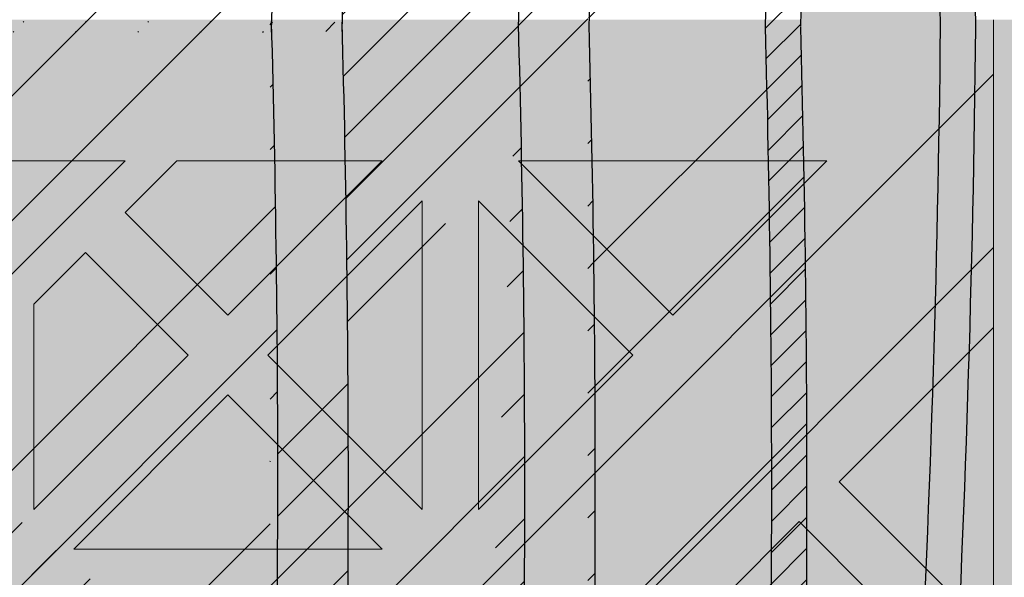
# Model space of a CAD drawing. Units: inches. Extents: x 844 to 2234, y 346 to 1084.
# Tile 54 of 93: x 1869.404 to 1873.853, y 698.846 to 701.365. Entities that reach past the tile are written whole.
import ezdxf

# ---------------------------------------------------------------- set-up
doc = ezdxf.new("R2010")
doc.units = ezdxf.units.IN
doc.header["$MEASUREMENT"] = 0
doc.layers.add('furniture', color=8, linetype='Continuous', lineweight=18)
doc.layers.add('RA-AP-01$0$INT', color=35, linetype='Continuous', lineweight=5)
doc.layers.add('RA-AP-01$0$FURN', color=3, linetype='Continuous')
doc.layers.add('RA-AP-01$0$WOOD', color=64, linetype='Continuous')

# ---------------------------------------------------------------- blocks, each defined once
blk = doc.blocks.new('A$C18D01794')
at = {"layer": 'RA-AP-01$0$INT'}
blk.add_hatch(color=256, dxfattribs=at).paths.add_polyline_path([(4.505206456958071, -6.306712009588038), (5.305206456958072, -6.306712009588038), (5.305206456958072, -7.106712009588038), (5.255206456951893, -7.10671200958804), (5.25520645694868, -6.356712009605972), (4.555206456959269, -6.356712009587461), (4.555206456956052, -7.106712009588038), (4.505206456958073, -7.106712009588038)])
h = blk.add_hatch(color=256, dxfattribs=at)
h.paths.add_polyline_path([(4.585917135068449, -6.356712009588271), (4.555206456959269, -6.35671200958746), (4.555206456959137, -6.387422687716308), (4.874495778835233, -6.706712009592356), (4.90520645695423, -6.676001331474049)])
h.paths.add_polyline_path([(5.255206456948813, -6.387422687716306), (5.255206456948682, -6.356712009605972), (5.224495778822613, -6.356712009605161), (4.905206456953498, -6.676001331474273), (4.935917135072151, -6.706712009592924)])
h.paths.add_polyline_path([(4.935917135072559, -6.706712009592068), (4.905206456953564, -6.737422687710376), (5.255206456951813, -7.087422687708613), (5.255206456951549, -7.026001331471008)])
h.paths.add_polyline_path([(4.555206456956399, -7.026001331471013), (4.555206456956134, -7.087422687708616), (4.905206456953821, -6.737422687710943), (4.874495778835166, -6.70671200959229)])
h = blk.add_hatch(color=256, dxfattribs=at)
h.paths.add_polyline_path([(4.585917135068448, -6.356712009588273), (4.614201406330596, -6.356712009589021), (4.668846067270487, -6.411356670531338), (4.723490728212344, -6.356712009591912), (4.771774999457151, -6.35671200959319), (4.826419660396886, -6.411356670535356), (4.862780050090322, -6.374996280843536), (4.844495778842715, -6.356712009595112), (4.862780050090411, -6.356712009595595), (4.905206456960182, -6.399138416468211), (4.947632863832445, -6.356712009597838), (4.965917135079675, -6.356712009598322), (4.947632863831759, -6.374996280845421), (4.983993253523576, -6.411356670538857), (5.038637914464627, -6.356712009600247), (5.08692218571208, -6.356712009601523), (5.141566846649976, -6.411356670541852), (5.196211507589851, -6.356712009604411), (5.224495778822615, -6.356712009605161), (4.905206456953975, -6.676001331473793)])
h.paths.add_polyline_path([(4.895206456956031, -6.637717060225675), (4.895206456958921, -6.528427738347902), (4.840561796018589, -6.583072399285802)], flags=16)
h.paths.add_polyline_path([(4.915206456955638, -6.637717060226121), (4.969851117895509, -6.583072399288678), (4.915206456957609, -6.528427738348344)], flags=16)
h.paths.add_polyline_path([(4.826419660395175, -6.568930263661755), (4.881064321335613, -6.514285602723745), (4.771774999456703, -6.514285602720857)], flags=16)
h.paths.add_polyline_path([(4.983993253519558, -6.568930263665262), (5.038637914460456, -6.514285602726792), (4.929348592581548, -6.514285602724816)], flags=16)
h.paths.add_polyline_path([(4.881064321336025, -6.494285602723742), (4.826419660397532, -6.439640941782821), (4.771774999457062, -6.494285602720859)], flags=16)
h.paths.add_polyline_path([(4.929348592582019, -6.494285602724817), (5.038637914460982, -6.494285602726792), (4.983993253522945, -6.439640941786327)], flags=16)
h.paths.add_polyline_path([(4.895206456960191, -6.480143467100443), (4.895206456962115, -6.407422687715913), (4.876922185715016, -6.389138416467584), (4.840561796021581, -6.425498806159401)], flags=16)
h.paths.add_polyline_path([(4.915206456958487, -6.480143467100889), (4.969851117899527, -6.425498806162279), (4.933490728206909, -6.389138416468043), (4.9152064569598, -6.40742268771434)], flags=16)
h.paths.add_polyline_path([(4.757632863832376, -6.480143467096812), (4.812277524772842, -6.425498806158772), (4.757632863834348, -6.370854145217844)], flags=16)
h.paths.add_polyline_path([(4.737632863832376, -6.480143467096286), (4.737632863834348, -6.370854145217375), (4.682988202893906, -6.425498806155385)], flags=16)
h.paths.add_polyline_path([(5.05278005008503, -6.480143467103376), (5.052780050087917, -6.370854145224413), (4.998135389146995, -6.425498806162908)], flags=16)
h.paths.add_polyline_path([(5.072780050085024, -6.480143467103744), (5.127424711025931, -6.42549880616527), (5.072780050087916, -6.370854145224832)], flags=16)
h.paths.add_polyline_path([(4.935917135072783, -6.706712009592292), (5.255206456948811, -6.387422687716309), (5.255206456948932, -6.415706958964177), (5.200561796010279, -6.470351619902839), (5.255206456949403, -6.524996280841948), (5.25520645694961, -6.5732805520894), (5.200561796009787, -6.627925213029239), (5.236922185702417, -6.664285602721864), (5.255206456949919, -6.646001331474357), (5.255206456949998, -6.664285602721898), (5.212780050078687, -6.706712009592262), (5.25520645695036, -6.749138416463932), (5.255206456950438, -6.767422687711313), (5.236922185702424, -6.749138416463297), (5.200561796009796, -6.785498806155928), (5.255206456950753, -6.840143467096874), (5.25520645695096, -6.888427738341682), (5.200561796010322, -6.943072399282328), (5.255206456951428, -6.997717060223427), (5.255206456951547, -7.026001331471006)])
h.paths.add_polyline_path([(5.042988202883395, -6.785498806155427), (5.097632863823085, -6.840143467095101), (5.097632863822622, -6.730854145216193)], flags=16)
h.paths.add_polyline_path([(5.028846067259663, -6.771356670531693), (5.083490728198774, -6.716712009592573), (4.974201406321001, -6.716712009593042)], flags=16)
h.paths.add_polyline_path([(5.117632863823087, -6.840143467095186), (5.172277524762331, -6.785498806155926), (5.11763286382262, -6.730854145216225)], flags=16)
h.paths.add_polyline_path([(5.08349072819877, -6.696712009593886), (5.028846067259652, -6.642067348654775), (4.974201406320998, -6.696712009593438)], flags=16)
h.paths.add_polyline_path([(5.131774999446817, -6.854285602718917), (5.186419660386065, -6.799640941779662), (5.241064321325782, -6.854285602719365)], flags=17)
h.paths.add_polyline_path([(5.131774999446228, -6.716712009592374), (5.186419660386065, -6.771356670532194), (5.222780050079488, -6.734996280838764), (5.204495778832781, -6.716712009592063)], flags=16)
h.paths.add_polyline_path([(5.097632863822613, -6.682569873970264), (5.097632863823061, -6.573280552091354), (5.042988202883383, -6.627925213031044)], flags=16)
h.paths.add_polyline_path([(5.131774999446899, -6.874285602718915), (5.241064321325809, -6.874285602719364), (5.186419660386591, -6.928930263658598)], flags=17)
h.paths.add_polyline_path([(5.131774999446226, -6.696712009594078), (5.204495778830767, -6.696712009594374), (5.22278005007868, -6.67842773834687), (5.186419660386049, -6.642067348654249)], flags=16)
h.paths.add_polyline_path([(5.11763286382262, -6.682569873970225), (5.17227752476232, -6.627925213030515), (5.117632863823064, -6.573280552091267)], flags=16)
h.paths.add_polyline_path([(5.186419660386069, -6.613783077405491), (5.241064321325754, -6.559138416465795), (5.131774999446791, -6.559138416466263)], flags=16)
h.paths.add_polyline_path([(5.131774999446872, -6.539138416466263), (5.24106432132578, -6.539138416465794), (5.186419660386554, -6.484493755526573)], flags=16)
h.paths.add_polyline_path([(5.255206456951811, -7.08742268770861), (5.255206456951895, -7.106712009588038), (4.555206456956052, -7.106712009588038), (4.555206456956136, -7.087422687708617), (4.905206456953973, -6.737422687710788)])
h.paths.add_polyline_path([(4.983993253513404, -6.8444937555241), (4.92934859257295, -6.899138416462108), (5.03863791445186, -6.899138416465014)], flags=16)
h.paths.add_polyline_path([(4.969851117889988, -6.83035161990006), (4.915206456952556, -6.775706958960171), (4.915206456949648, -6.884996280837944)], flags=16)
h.paths.add_polyline_path([(4.929348592572535, -6.919138416462105), (4.983993253511019, -6.973783077403037), (5.038637914451496, -6.919138416465012)], flags=16)
h.paths.add_polyline_path([(5.052780050074912, -6.93328055208906), (4.998135389134438, -6.987925213027088), (5.052780050072919, -7.042569873968025)], flags=16)
h.paths.add_polyline_path([(5.07278005007491, -6.933280552089588), (5.072780050072918, -7.042569873968497), (5.127424711013374, -6.987925213030498)], flags=16)
h.paths.add_polyline_path([(4.89520645695295, -6.775706958959721), (4.840561796013067, -6.830351619897157), (4.895206456950961, -6.884996280837494)], flags=16)
h.paths.add_polyline_path([(4.915206456948365, -6.933280552085403), (4.915206456946434, -7.006001331471951), (4.933490728192729, -7.024285602719066), (4.969851117886972, -6.987925213026453)], flags=16)
h.paths.add_polyline_path([(4.881064321327021, -6.899138416461022), (4.82641966038902, -6.84449375552057), (4.771774999448108, -6.899138416459029)], flags=16)
h.paths.add_polyline_path([(4.895206456950073, -6.933280552084951), (4.840561796009022, -6.987925213023558), (4.876922185700835, -7.024285602716997), (4.895206456948749, -7.006001331469487)], flags=16)
h.paths.add_polyline_path([(4.983993253510392, -7.0020673486505), (4.947632863816944, -7.038427738342319), (4.965917135064043, -7.05671200959023), (5.038637914448995, -7.056712009591555)], flags=16)
h.paths.add_polyline_path([(4.881064321326543, -6.91913841646102), (4.771774999447578, -6.919138416459031), (4.826419660385607, -6.973783077399508)], flags=16)
h.paths.add_polyline_path([(4.905206456946447, -7.014285602717636), (4.862780050074785, -7.056712009588352), (4.947632863816685, -7.056712009589775)], flags=16)
h.paths.add_polyline_path([(5.14156684663679, -7.002067348654549), (5.086922185696452, -7.056712009592438), (5.196211507574223, -7.056712009594425)], flags=16)
h.paths.add_polyline_path([(4.8264196603837, -7.002067348646972), (4.771774999442643, -7.056712009585575), (4.8444957788276, -7.056712009587508), (4.862780050075511, -7.038427738340416)], flags=16)
h.paths.add_polyline_path([(4.812277524760289, -6.98792521302292), (4.757632863822258, -6.933280552082447), (4.757632863819352, -7.042569873961408)], flags=16)
h.paths.add_polyline_path([(4.73763286382226, -6.933280552082079), (4.682988202881349, -6.987925213020536), (4.737632863819352, -7.04256987396099)], flags=16)
h.paths.add_polyline_path([(4.723490728195188, -7.056712009584289), (4.668846067257299, -7.002067348643949), (4.614201406317417, -7.056712009581383)], flags=16)
h.paths.add_polyline_path([(4.597632863829262, -6.706712009592262), (4.555206456957951, -6.664285602721896), (4.555206456958029, -6.646001331474357), (4.573490728205535, -6.664285602721864), (4.609851117898167, -6.627925213029238), (4.555206456958338, -6.573280552089402), (4.555206456958546, -6.524996280841952), (4.60985111789767, -6.470351619902839), (4.555206456959015, -6.415706958964177), (4.555206456959138, -6.387422687716309), (4.874495778835167, -6.70671200959229), (4.5552064569564, -7.026001331471015), (4.555206456956523, -6.997717060223433), (4.609851117897629, -6.94307239928233), (4.555206456956988, -6.888427738341681), (4.555206456957198, -6.840143467096881), (4.609851117898153, -6.78549880615593), (4.573490728205528, -6.749138416463297), (4.555206456957507, -6.76742268771132), (4.555206456957585, -6.749138416463933)])
h.paths.add_polyline_path([(4.712780050085332, -6.730854145216195), (4.712780050084863, -6.840143467095105), (4.767424711024555, -6.785498806155427)], flags=16)
h.paths.add_polyline_path([(4.726922185709173, -6.716712009592573), (4.781566846648288, -6.771356670531693), (4.836211507586949, -6.716712009593043)], flags=16)
h.paths.add_polyline_path([(4.692780050085327, -6.730854145216225), (4.638135389145619, -6.785498806155928), (4.692780050084865, -6.840143467095185)], flags=16)
h.paths.add_polyline_path([(4.726922185709182, -6.696712009593886), (4.836211507586949, -6.696712009593436), (4.7815668466483, -6.642067348654773)], flags=16)
h.paths.add_polyline_path([(4.678637914461726, -6.71671200959237), (4.605917135075169, -6.716712009592063), (4.587632863828464, -6.734996280838766), (4.623993253521887, -6.771356670532195)], flags=16)
h.paths.add_polyline_path([(4.712780050085336, -6.68256987397026), (4.767424711024568, -6.627925213031042), (4.71278005008489, -6.573280552091352)], flags=16)
h.paths.add_polyline_path([(4.678637914461726, -6.696712009594076), (4.623993253521899, -6.642067348654247), (4.587632863829271, -6.67842773834687), (4.605917135077185, -6.696712009594376)], flags=16)
h.paths.add_polyline_path([(4.692780050085336, -6.682569873970228), (4.692780050084889, -6.573280552091267), (4.638135389145632, -6.627925213030515)], flags=16)
h.paths.add_polyline_path([(4.623993253521885, -6.799640941779662), (4.678637914461131, -6.854285602718915), (4.56934859258217, -6.854285602719365)], flags=17)
h.paths.add_polyline_path([(4.623993253521901, -6.613783077405509), (4.678637914461158, -6.559138416466263), (4.569348592582195, -6.559138416465795)], flags=16)
h.paths.add_polyline_path([(4.678637914461051, -6.874285602718915), (4.623993253521361, -6.928930263658598), (4.569348592582143, -6.874285602719364)], flags=17)
h.paths.add_polyline_path([(4.678637914461076, -6.539138416466263), (4.623993253521399, -6.484493755526573), (4.569348592582167, -6.539138416465796)], flags=16)
h = blk.add_hatch(color=256, dxfattribs=at)
h.paths.add_polyline_path([(5.028846067259997, -6.642067348655121), (4.974201406321342, -6.696712009593783), (5.083490728199115, -6.69671200959423)])
h.paths.add_polyline_path([(4.974201406321344, -6.716712009593388), (5.028846067260004, -6.771356670532039), (5.083490728199117, -6.716712009592919)])
h.paths.add_polyline_path([(5.042988202883738, -6.785498806155768), (5.097632863823428, -6.840143467095449), (5.097632863822963, -6.73085414521654)])
h.paths.add_polyline_path([(5.117632863822961, -6.730854145216568), (5.117632863823428, -6.840143467095531), (5.172277524762674, -6.785498806156272)])
h.paths.add_polyline_path([(5.131774999446572, -6.716712009592718), (5.186419660386406, -6.77135667053254), (5.222780050079831, -6.734996280839116), (5.204495778833122, -6.716712009592409)])
h.paths.add_polyline_path([(5.236922185702764, -6.749138416463644), (5.200561796010139, -6.785498806156274), (5.255206456949971, -6.840143467096101), (5.255206456950271, -6.76742268771115)])
h.paths.add_polyline_path([(5.186419660386412, -6.799640941780006), (5.131774999447164, -6.854285602719262), (5.241064321326123, -6.854285602719711)])
h.paths.add_polyline_path([(5.131774999447238, -6.874285602719261), (5.186419660386934, -6.928930263658944), (5.241064321326153, -6.874285602719709)])
h.paths.add_polyline_path([(5.200561796010663, -6.943072399282675), (5.255206456949324, -6.997717060221329), (5.255206456949777, -6.888427738343558)])
h.paths.add_polyline_path([(5.21278005007903, -6.706712009592607), (5.255206456950223, -6.749138416463798), (5.255206456950696, -6.664285602721891)])
h.paths.add_polyline_path([(5.13177499944657, -6.696712009594424), (5.204495778831106, -6.696712009594723), (5.222780050079024, -6.678427738347219), (5.186419660386397, -6.642067348654592)])
h.paths.add_polyline_path([(5.117632863823405, -6.573280552091611), (5.117632863822955, -6.682569873970578), (5.172277524762665, -6.627925213030859)])
h.paths.add_polyline_path([(5.042988202883727, -6.627925213031387), (5.097632863822957, -6.682569873970603), (5.097632863823407, -6.573280552091697)])
h.paths.add_polyline_path([(5.131774999447135, -6.559138416466609), (5.186419660386394, -6.613783077405857), (5.241064321326097, -6.559138416466144)])
h.paths.add_polyline_path([(5.200561796010128, -6.627925213029584), (5.236922185702758, -6.664285602722211), (5.255206456950264, -6.646001331474705), (5.255206456949948, -6.573280552089752)])
h.paths.add_polyline_path([(5.186419660386895, -6.484493755526919), (5.131774999447213, -6.539138416466609), (5.241064321326127, -6.539138416466142)])
h.paths.add_polyline_path([(5.200561796010624, -6.470351619903183), (5.255206456949745, -6.524996280842298), (5.255206456949276, -6.415706958964523)])
h = blk.add_hatch(color=256, dxfattribs=at)
h.paths.add_polyline_path([(4.895206456952951, -6.77570695895972), (4.840561796013068, -6.830351619897156), (4.895206456950958, -6.884996280837495)])
h.paths.add_polyline_path([(4.915206456949649, -6.884996280837942), (4.969851117889987, -6.830351619900054), (4.915206456952556, -6.775706958960171)])
h.paths.add_polyline_path([(5.038637914451862, -6.899138416465013), (4.983993253513403, -6.8444937555241), (4.929348592572953, -6.899138416462106)])
h.paths.add_polyline_path([(4.929348592572535, -6.919138416462105), (4.983993253511018, -6.973783077403037), (5.038637914451497, -6.919138416465012)])
h.paths.add_polyline_path([(4.915206456948366, -6.933280552085397), (4.915206456946433, -7.006001331471951), (4.93349072819273, -7.024285602719068), (4.969851117886972, -6.987925213026454)])
h.paths.add_polyline_path([(5.038637914448995, -7.056712009591553), (4.983993253510389, -7.002067348650502), (4.947632863816946, -7.038427738342318), (4.965917135064043, -7.05671200959023)])
h.paths.add_polyline_path([(5.05278005007292, -7.042569873968023), (5.05278005007491, -6.933280552089059), (4.998135389134438, -6.987925213027088)])
h.paths.add_polyline_path([(5.07278005007292, -7.042569873968496), (5.127424711013374, -6.987925213030498), (5.072780050074909, -6.933280552089588)])
h.paths.add_polyline_path([(5.141566846636789, -7.002067348654547), (5.086922185696449, -7.056712009592438), (5.196211507574223, -7.056712009594425)])
h.paths.add_polyline_path([(4.947632863816688, -7.056712009589774), (4.905206456946449, -7.014285602717634), (4.862780050074784, -7.056712009588353)])
h.paths.add_polyline_path([(4.840561796009025, -6.987925213023556), (4.876922185700834, -7.024285602716997), (4.895206456948747, -7.006001331469488), (4.895206456950075, -6.933280552084953)])
h.paths.add_polyline_path([(4.88106432132654, -6.919138416461021), (4.771774999447577, -6.919138416459031), (4.826419660385606, -6.973783077399508)])
h.paths.add_polyline_path([(4.881064321327019, -6.899138416461022), (4.826419660389019, -6.844493755520571), (4.771774999448108, -6.89913841645903)])
h.paths.add_polyline_path([(4.757632863819352, -7.042569873961409), (4.812277524760284, -6.987925213022922), (4.757632863822259, -6.933280552082447)])
h.paths.add_polyline_path([(4.8264196603837, -7.002067348646974), (4.771774999442646, -7.056712009585575), (4.844495778827599, -7.05671200958751), (4.862780050075512, -7.038427738340417)])
h.paths.add_polyline_path([(4.737632863819352, -7.042569873960988), (4.737632863822258, -6.933280552082078), (4.682988202881349, -6.987925213020538)])
h.paths.add_polyline_path([(4.668846067257299, -7.002067348643952), (4.61420140631742, -7.056712009581384), (4.723490728195189, -7.056712009584292)])
for p, q in [((5.255206456951895, -7.106712009588038), (5.255206456948681, -6.356712009605972)), ((4.935917135072783, -6.706712009592292), (5.255206456951548, -7.026001331471007)), ((4.905206456953975, -6.737422687710788), (5.255206456951811, -7.087422687708611)), ((5.186419660386587, -6.928930263658596), (5.131774999446899, -6.874285602718915)), ((5.241064321325809, -6.874285602719364), (5.186419660386589, -6.928930263658598)), ((5.255206456949429, -6.888427738343214), (5.200561796010322, -6.943072399282328)), ((5.255206456949433, -6.888427738343212), (5.255206456948982, -6.997717060220983)), ((5.038637914451498, -6.919138416465012), (4.929348592572535, -6.919138416462105)), ((4.929348592572535, -6.919138416462105), (4.983993253511019, -6.973783077403037)), ((5.038637914451498, -6.919138416465012), (4.983993253511019, -6.973783077403037)), ((4.915206456946434, -7.006001331470351), (4.915206456948367, -6.933280552085399)), ((4.915206456948367, -6.933280552085399), (4.969851117886972, -6.987925213026453)), ((5.05278005007491, -6.93328055208906), (4.998135389134438, -6.987925213027088)), ((5.05278005007491, -6.93328055208906), (5.052780050072921, -7.042569873968023)), ((5.127424711013373, -6.987925213030496), (5.07278005007491, -6.933280552089588)), ((5.07278005007491, -6.933280552089588), (5.07278005007292, -7.042569873968497)), ((5.255206456948982, -6.997717060220983), (5.200561796010322, -6.943072399282328)), ((4.969851117886972, -6.987925213026452), (4.93349072819353, -7.024285602718265)), ((5.052780050072921, -7.042569873968023), (4.998135389134438, -6.987925213027088)), ((5.07278005007292, -7.042569873968497), (5.127424711013374, -6.987925213030498)), ((4.98399325351039, -7.002067348650502), (4.947632863816946, -7.038427738342317)), ((5.038637914448995, -7.056712009591555), (4.983993253510388, -7.002067348650502)), ((5.086922185696454, -7.056712009592434), (5.141566846636789, -7.002067348654547)), ((5.196211507574223, -7.056712009594425), (5.141566846636789, -7.002067348654547)), ((4.915206456946427, -7.006001331471944), (4.933490728193524, -7.02428560271986)), ((4.905206456946449, -7.014285602717635), (4.94763286381669, -7.056712009589775)), ((4.947632863816946, -7.038427738342317), (4.965917135063997, -7.056712009590183)), ((4.965917135064043, -7.056712009590231), (4.947632863816944, -7.038427738342317)), ((4.94763286381669, -7.056712009589775), (4.862780050074783, -7.056712009588354)), ((4.965917135064043, -7.05671200959023), (5.038637914448995, -7.056712009591555)), ((5.086922185696452, -7.056712009592438), (5.196211507574223, -7.056712009594425))]:
    blk.add_line(p, q, dxfattribs=at)
blk = doc.blocks.new('A$C32926AE1')
at = {"layer": 'RA-AP-01$0$FURN'}
h = blk.add_hatch(dxfattribs=at)
h.set_pattern_fill('ANSI31', color=256, scale=0.1, style=0)
h.set_pattern_definition([(45, (0, 0), (-0.0088388347648318, 0.0088388347648318), [])])
edge = h.paths.add_edge_path(flags=16)
edge.add_arc((4.904771284329206, 4.246793130718756), 0.2603971832811541, 75.22398030683196, 104.7760196931204)
edge.add_arc((4.904771284329206, 4.246793130718756), 0.2603971832811541, 75.223980306832, 104.77601969312039, ccw=False)
edge = h.paths.add_edge_path(flags=16)
edge.add_arc((4.904771284329206, 4.067062675376612), 0.2603971832811541, 255.2239803068796, 284.776019693168)
edge.add_arc((4.904771284329206, 4.067062675376612), 0.2603971832811541, 255.22398030687958, 284.77601969316805, ccw=False)
edge = h.paths.add_edge_path(flags=0)
edge.add_arc((4.904771284329206, 4.067062675376612), 0.2603971832811541, 255.2239803068796, 284.776019693168)
edge.add_arc((4.904771284329206, 4.067062675376612), 0.2603971832811541, 255.22398030687958, 284.77601969316805, ccw=False)
edge = h.paths.add_edge_path(flags=0)
edge.add_arc((4.904771284329206, 4.067062675376612), 0.2603971832811541, 255.2239803068796, 284.776019693168)
edge.add_arc((4.904771284329206, 4.067062675376612), 0.2603971832811541, 255.22398030687958, 284.77601969316805, ccw=False)
edge = h.paths.add_edge_path()
edge.add_arc((4.604388392048174, 4.588829985554312), 0.1599999999999918, 342.3781640246255, 354.4317409793762)
edge.add_arc((5.090145208887507, 4.43216705527679), 0.3503971832811637, 162.0091218307731, 180.3186872093483)
edge.add_arc((5.205154176610243, 4.588829985554953), 0.1599999999999917, 185.5682590208461, 197.6218359767349)
edge.add_arc((4.904771284329229, 4.246793130718735), 0.3503971832811761, 72.00912183053516, 107.9908781690354)
edge.add_arc((9.535952835716557, 4.28682295566602), 4.798342501046485, 178.2875002453811, 181.5576802719453)
edge.add_arc((4.719397359771122, 4.43216705527679), 0.3503971832811637, 359.6813127906516, 377.9908781692269)
edge.add_arc((9.535967292294904, 4.286822350292874), 4.778371420254705, 178.2965938931842, 181.5667745797229)
edge.add_arc((4.719397359771122, 4.43216705527679), 0.3303971832811637, 359.6813127906516, 377.9908781692269)
edge.add_arc((0.2735752763637294, 4.286822350292874), 4.7783714202547, 358.4332254202771, 361.7034061068158)
edge.add_arc((5.061434214606998, 4.732549947558029), 0.1600000000000254, 252.3781640250584, 264.4317409792362)
edge.add_arc((4.748108354051257, 4.732549947558012), 0.1600000000000541, 275.5682590208426, 287.6218359759532)
edge.add_arc((4.604388392048115, 4.588829985554317), 0.1800000000000505, 342.3567572500182, 349.3735009646207)
edge.add_arc((5.205154176610254, 4.588829985554976), 0.1800000000000069, 190.6264990356027, 197.6432427513933)
edge.add_arc((5.061434214607106, 4.732549947558013), 0.1800000000000424, 252.3567572496606, 259.3735009644582)
edge.add_arc((4.904771284329208, 4.246793130718737), 0.3303971832811676, 71.99844483668534, 108.0015551637021)
edge.add_arc((4.748108354051414, 4.732549947558045), 0.1800000000000547, 280.6264990355479, 287.6432427495938)
edge.add_arc((5.090145208887514, 4.432167055276789), 0.2803971832811691, 162.8706300666893, 180.816523289902)
edge.add_arc((4.719397359771136, 4.432167055276689), 0.2803971832811534, 359.183476710103, 377.1293699333214)
edge.add_arc((4.904771284329222, 4.246793130718737), 0.2803971832811769, 72.87063006672916, 107.1293699332334)
edge.add_arc((5.090145208887522, 4.432167055276788), 0.2603971832811776, 165.2239803068007, 180.9953123810312)
edge.add_arc((4.719397359771141, 4.432167055276699), 0.2603971832811458, 359.0046876189768, 374.7760196932087)
edge.add_arc((5.090145208887507, 4.43216705527679), 0.3303971832811637, 162.0091218307731, 180.3186872093483)
edge.add_arc((9.53595427642584, 4.285015535491528), 4.728345371032053, 178.265043920078, 181.5679956281801)
edge.add_arc((0.2735882922327999, 4.285015535491582), 4.728345371032045, 358.4320043718193, 361.7349560799204)
edge.add_arc((9.535953591267507, 4.284458026472751), 4.708343996644348, 178.2573054306777, 181.5704995759608)
edge.add_arc((0.273588977391114, 4.284458026472785), 4.708343996644358, 358.4295004240388, 361.7426945693213)
edge.add_arc((0.2735889773911131, 4.029397779622582), 4.708343996644359, 358.2573054306787, 361.5704995759613)
edge.add_arc((9.535953591267518, 4.029397779622618), 4.708343996644359, 178.4295004240391, 181.7426945693223)
edge.add_arc((0.2735882922327901, 4.028840270603786), 4.728345371032054, 358.2650439200796, 361.5679956281808)
edge.add_arc((9.53595427642584, 4.028840270603841), 4.728345371032054, 178.4320043718199, 181.7349560799219)
edge.add_arc((0.2735752763637302, 4.027033455802493), 4.778371420254699, 358.2965938931842, 361.5667745797229)
edge.add_arc((4.719397359771122, 3.881688750818578), 0.3303971832811637, 342.0091218307731, 360.3186872093484)
edge.add_arc((5.090145208887507, 3.881688750818578), 0.3303971832811637, 179.6813127906516, 197.9908781692269)
edge.add_arc((9.535967292294904, 4.027033455802493), 4.778371420254705, 178.433225420277, 181.7034061068158)
edge.add_arc((4.719397359771122, 3.881688750818578), 0.3503971832811637, 342.0091218307731, 360.3186872093484)
edge.add_arc((9.53595283571655, 4.027032850429349), 4.79834250104648, 178.4423197280546, 181.7124997546188)
edge.add_arc((4.719397359771141, 3.881688750818669), 0.2603971832811458, 345.2239803067913, 360.9953123810232)
edge.add_arc((5.090145208887522, 3.88168875081858), 0.2603971832811776, 179.0046876189687, 194.7760196931993)
edge.add_arc((4.904771284329222, 4.067062675376631), 0.2803971832811769, 252.8706300667665, 287.1293699332708)
edge.add_arc((4.719397359771136, 3.881688750818678), 0.2803971832811534, 342.8706300666787, 360.8165232898969)
edge.add_arc((5.090145208887514, 3.881688750818579), 0.2803971832811691, 179.183476710098, 197.1293699333106)
edge.add_arc((4.748108354051414, 3.581305858537323), 0.1800000000000547, 72.3567572504062, 79.37350096445199)
edge.add_arc((4.904771284329208, 4.067062675376631), 0.3303971832811676, 251.9984448362979, 288.0015551633146)
edge.add_arc((5.061434214607106, 3.581305858537355), 0.1800000000000424, 100.6264990355418, 107.6432427503394)
edge.add_arc((5.205154176610254, 3.725025820540392), 0.1800000000000069, 162.3567572486066, 169.3735009643972)
edge.add_arc((4.604388392048115, 3.725025820541051), 0.1800000000000505, 10.62649903537925, 17.64324274998182)
edge.add_arc((4.748108354051257, 3.581305858537356), 0.1600000000000541, 72.37816402404681, 84.43174097915735)
edge.add_arc((4.904771284329229, 4.067062675376632), 0.3503971832811761, 252.0091218309645, 287.9908781694648)
edge.add_arc((5.061434214606998, 3.581305858537339), 0.1600000000000254, 95.56825902076373, 107.6218359749416)
edge.add_arc((5.205154176610243, 3.725025820540414), 0.1599999999999917, 162.3781640232651, 174.4317409791539)
edge.add_arc((5.090145208887507, 3.881688750818578), 0.3503971832811637, 179.6813127906516, 197.9908781692269)
edge.add_arc((4.604388392048174, 3.725025820541056), 0.1599999999999918, 5.568259020623824, 17.62183597537444)
edge.add_arc((0.2735897329420762, 4.28682295566602), 4.798342501046482, 358.4423197280547, 361.7124997546188)
edge.add_arc((0.2735897329420691, 4.027032850429348), 4.798342501046489, 358.2875002453812, 361.5576802719453)
at = {"layer": 'RA-AP-01$0$WOOD'}
h = blk.add_hatch(color=256, dxfattribs=at)
h.dxf.hatch_style = 1
h.paths.add_polyline_path([(5.157430609644524, 4.573483066760929, -0.1009492694046607), (5.155401577623758, 4.593365984175333, -0.1842662638101597), (5.172249623284174, 4.638795604568598, 0.2056608120311276), (5.179560981299304, 4.661316324430096, 0.3614336704623542), (5.134352340494423, 4.706524965234944, 0.2056608120311297), (5.111831620632933, 4.699213607219793, -0.1842662638101113), (5.066402000239693, 4.682365561559342, -0.1055311479399994), (5.045656153913092, 4.68467289944697, 0.1567636581983829), (4.763886414745334, 4.684672899446966, -0.1055311479399895), (4.743140568418733, 4.68236556155934, -0.1842662638100833), (4.6977109480255, 4.69921360721979, 0.2056608120302612), (4.675190228164109, 4.706524965234949, 0.3614336704708441), (4.629981587358889, 4.66131632442871, 0.2056608120245944), (4.637292945374126, 4.638795604567974, -0.1842662638101024), (4.654140991034615, 4.59336598417475, -0.1009492694055169), (4.652111959013835, 4.573483066760181, 0.021410119221476), (4.629748025606143, 4.156712009541676, 0.0214101192214795), (4.652111959013809, 3.739940952323101, -0.1009492694059586), (4.654140991034615, 3.720058034908448, -0.1842662638100975), (4.637292945374126, 3.674628414515226, 0.2056608120245705), (4.629981587358889, 3.652107694654492, 0.3614336704708879), (4.675190228164113, 3.606899053848249, 0.2056608120302384), (4.697710948025501, 3.614210411863408, -0.1842662638100995), (4.743140568418738, 3.63105845752386, -0.1055311479402541), (4.763886414745388, 3.628751119636215, 0.1567636581983776), (5.045656153913137, 3.628751119636244, -0.1055311479397538), (5.066402000239692, 3.631058457523857, -0.1842662638101067), (5.111831620632931, 3.614210411863407, 0.2056608120310924), (5.134352340494417, 3.606899053848256, 0.3614336704624001), (5.179560981299307, 3.652107694653103, 0.2056608120311314), (5.172249623284175, 3.6746284145146, -0.1842662638101402), (5.155401577623758, 3.72005803490786, -0.1009492694051366), (5.15743060964455, 3.739940952322354, 0.0214101192215073), (5.179794543052287, 4.156712009541468, 0.0214101192215252)])
h.paths.add_polyline_path([(4.639748609479751, 4.156712009541513, 0.0213537860821624), (4.661970494867118, 3.741887061152232, -0.094075836301374), (4.664143710413708, 3.7196126951003, -0.1824818158568985), (4.644813765429836, 3.668037719127816, 0.2056608120245319), (4.639939526753007, 3.653023905887301, 0.3614336704710246), (4.676106439397173, 3.616856993242342, 0.2056608120302234), (4.691120252638095, 3.621731231919122, -0.1824818158602558), (4.742695228611606, 3.641061176902986, -0.1029891339458722), (4.766991894714349, 3.638256818950944, 0.156709409989566), (5.042550673941472, 3.638256818950105, -0.102989133958497), (5.066847340047078, 3.641061176902949, -0.1824818158594995), (5.118422316020358, 3.621731231919103, 0.2056608120311416), (5.133436129261316, 3.616856993242346, 0.3614336704621468), (5.169603041905217, 3.653023905886178, 0.2056608120310986), (5.164728803228477, 3.668037719127177, -0.1824818158565612), (5.145398858244737, 3.719612695099578, -0.0940758363009313), (5.147572073791232, 3.741887061151398, 0.0213537860822023), (5.169793959178681, 4.156712009541451, 0.0213537860822226), (5.147572073791203, 4.571536957931898, -0.0940758363005034), (5.145398858244737, 4.59381132398362, -0.1824818158565587), (5.164728803228476, 4.645386299956021, 0.2056608120311045), (5.169603041905216, 4.66040011319702, 0.3614336704621845), (5.133436129261313, 4.696567025840856, 0.2056608120310773), (5.118422316020359, 4.691692787164098, -0.182481815859508), (5.066847340047078, 4.67236284218025, -0.1029891339584606), (5.04255067394148, 4.675167200133092, 0.156709409989566), (4.766991894714357, 4.675167200132257, -0.1029891339458842), (4.742695228611611, 4.672362842180213, -0.1824818158602725), (4.691120252638095, 4.691692787164077, 0.2056608120302152), (4.676106439397174, 4.696567025840858, 0.3614336704710363), (4.639939526753005, 4.660400113195899, 0.2056608120245495), (4.644813765429837, 4.645386299955384, -0.1824818158568934), (4.664143710413708, 4.593811323982902, -0.0940758363009187), (4.661970494867149, 4.571536957931074, 0.021353786082177)], flags=16)
h.paths.add_polyline_path([(5.129794543052235, 4.432167055276933, -0.0141661062790638), (5.130152669293814, 4.156927903047693, -0.0141661062790647), (5.129794543052234, 3.881688750818433, -0.0785247771143638), (5.10979738006795, 3.755143611847103, 0.0945969212073497), (5.105408519571111, 3.717898134952927, 0.1043170707844957), (5.116074640131521, 3.670385395016088, 0.1043170707864965), (5.068561900193738, 3.681051515576561, 0.09459692119553), (5.031316423304057, 3.676662655080835, -0.1580239521427272), (4.778226145355827, 3.676662655080367, 0.0945969211986668), (4.740980668464973, 3.681051515576592, 0.1043170707882822), (4.693467928526415, 3.670385395015844, 0.1043170707867916), (4.704134049087309, 3.717898134953662, 0.0945969211972894), (4.69974518859162, 3.755143611844042, -0.0785247771163196), (4.679748025606343, 3.881688750818406, -0.0141661062790663), (4.679389899364763, 4.156927903047693, -0.0141661062790672), (4.679748025606343, 4.432167055276998, -0.0785247771163064), (4.699745188591625, 4.55871219425134, 0.094596921197333), (4.704134049087308, 4.595957671141738, 0.1043170707867205), (4.693467928526416, 4.643470411079523, 0.1043170707882628), (4.740980668464965, 4.632804290518776, 0.0945969211988114), (4.778226145355874, 4.637193151015016, -0.158023952142669), (5.031316423304015, 4.637193151014546, 0.0945969211956361), (5.068561900193736, 4.632804290518806, 0.1043170707864979), (5.11607464013152, 4.643470411079278, 0.1043170707844617), (5.105408519571112, 4.595957671142455, 0.0945969212074597), (5.109797380067959, 4.558712194248236, -0.0785247771143467)], flags=0)
h.paths.add_polyline_path([(5.119794532311105, 4.432259799204851, -0.0142000800617244), (5.120156169157484, 4.156927903047701, -0.0142000800617277), (5.119794532311105, 3.881596006890482, -0.0784894509520253), (5.100273383573699, 3.758192358677797, 0.0940138827242913), (5.095413455884425, 3.717477693979438, 0.0606271852308753), (5.099615656341024, 3.686844378806616, 0.0606271852322524), (5.068982341167493, 3.691046579263239, 0.0940138827010453), (5.028267676478798, 3.686186651576848, -0.1580706864508061), (4.781274892180912, 3.686186651576435, 0.0940138827026903), (4.740560227491556, 3.691046579263279, 0.0606271852339895), (4.709926912317155, 3.686844378806508, 0.0606271852329405), (4.714129112773991, 3.717477693980356, 0.094013882701304), (4.709269185087677, 3.758192358669163, -0.0784894509577193), (4.689748036347473, 3.881596006890469, -0.014200080061729), (4.689386399501094, 4.156927903047709, -0.0142000800617217), (4.689748036347473, 4.432259799204808, -0.078489450957724), (4.709269185087651, 4.555663447426125, 0.0940138827014585), (4.714129112773992, 4.596378112114996, 0.0606271852329731), (4.709926912317154, 4.62701142728886, 0.0606271852340196), (4.74056022749157, 4.622809226832087, 0.0940138827024997), (4.781274892180847, 4.627669154518912, -0.1580706864508359), (5.028267676478777, 4.627669154518526, 0.0940138827010946), (5.068982341167492, 4.622809226832129, 0.060627185232254), (5.099615656341024, 4.627011427288751, 0.0606271852308727), (5.095413455884425, 4.59637811211593, 0.0940138827241088), (5.100273383573675, 4.555663447417647, -0.0784894509520978)], flags=0)
h.paths.add_polyline_path([(5.06978912287499, 4.430218106756144, -0.014241683694547), (5.070173729147532, 4.156927903047672, -0.0142416836945458), (5.06978912287499, 3.883637699339223, -0.0800609523125196), (5.052662118612511, 3.773463122773442, 0.0526421978001116), (5.04590916754064, 3.740550867606997, 0.0526421977992423), (5.012996912374707, 3.73379791653534, -0.1583028414718258), (4.796545656286308, 3.73379791653451, 0.0526421978034211), (4.763633401117837, 3.740550867607021, 0.0526421978018622), (4.756880450045755, 3.773463122774558, -0.0800609523117106), (4.739753445783639, 3.883637699339268, -0.0142416836945435), (4.739368839511098, 4.156927903047671, -0.0142416836945477), (4.739753445783639, 4.430218106756155, -0.0800609523116345), (4.75688045004574, 4.540392683320762, 0.052642197801941), (4.763633401117837, 4.573304938488346, 0.0526421978035071), (4.796545656286361, 4.580057889560873, -0.1583028414717561), (5.012996912374669, 4.580057889560039, 0.0526421977993048), (5.04590916754064, 4.57330493848837, 0.0526421978002057), (5.052662118612529, 4.540392683321868, -0.080060952312477)], flags=0)
h.paths.add_polyline_path([(5.049789715110557, 4.43038092723357, -0.0143097550741839), (5.05018085590259, 4.156927903047715, -0.0143097550741854), (5.049789715110558, 3.883474878861827, -0.0800685599149176), (5.03362098255317, 3.779581877367999, 0.0306258898956367), (5.028241146483733, 3.758218888663947, 0.0306258898977031), (5.006878157778253, 3.75283905259408, -0.1583983521624096), (4.802664410878162, 3.752839052594731, 0.0306258898946014), (4.781301422174808, 3.758218888663924, 0.0306258898967912), (4.775921586105202, 3.779581877368794, -0.080068559914251), (4.759752853548071, 3.883474878861786, -0.0143097550741854), (4.759361712756037, 4.156927903047671, -0.0143097550741854), (4.759752853548071, 4.430380927233557, -0.0800685599142479), (4.775921586105193, 4.534273928726546, 0.0306258898968306), (4.781301422174808, 4.555636917431444, 0.0306258898945754), (4.802664410878143, 4.561016753500631, -0.1583983521624168), (5.006878157778244, 4.561016753501291, 0.0306258898977177), (5.028241146483733, 4.555636917431421, 0.0306258898958182), (5.03362098255321, 4.534273928727244, -0.080068559914796)], flags=0)
h.paths.add_polyline_path([(4.999766070382627, 4.428171244713864, -0.0143443147609634), (5.000198441819402, 4.156927903047689, -0.0143443147609612), (4.999766070382627, 3.885684561381556, -0.0784641635803329), (4.987356730658798, 3.799103304488872, -0.1506053783831347), (4.822185837999821, 3.79910330448882, -0.0784641635803318), (4.809776498276007, 3.885684561381509, -0.014344314760963), (4.809344126839227, 4.156927903047677, -0.0143443147609645), (4.809776498276007, 4.428171244713873, -0.0784641635803192), (4.822185837999822, 4.514752501606549, -0.1506053783831338), (4.987356730658798, 4.514752501606494, -0.078464163580285)], flags=0)
h.paths.add_polyline_path([(4.979755254238824, 4.42764379880488, -0.0143772539198268), (4.980205517789977, 4.156927903047693, -0.0143772539198275), (4.979755254238824, 3.886212007290489, -0.0689242507424422), (4.971183264704897, 3.815276770442801, -0.1296645318904179), (4.838359303953726, 3.815276770442746, -0.0689242507424186), (4.829787314419809, 3.886212007290419, -0.0143772539198292), (4.829337050868653, 4.156927903047653, -0.0143772539198325), (4.829787314419809, 4.427643798804946, -0.0689242507424211), (4.838359303953725, 4.498579035652621, -0.1296645318904187), (4.971183264704897, 4.498579035652565, -0.0689242507424401)], flags=0)
h = blk.add_hatch(color=256, dxfattribs=at)
h.dxf.hatch_style = 1
h.paths.add_polyline_path([(5.145398858244737, 4.59381132398362, -0.1824818158565616), (5.164728803228476, 4.645386299956021, 0.2056608120311045), (5.169603041905216, 4.66040011319702, 0.3614336704621845), (5.133436129261313, 4.696567025840856, 0.2056608120310773), (5.118422316020359, 4.691692787164098, -0.182481815859508), (5.066847340047078, 4.67236284218025, -0.1029891339584606), (5.04255067394148, 4.675167200133092, 0.156709409989566), (4.766991894714357, 4.675167200132257, -0.1029891339458842), (4.742695228611611, 4.672362842180213, -0.1824818158602725), (4.691120252638095, 4.691692787164077, 0.2056608120302152), (4.676106439397174, 4.696567025840858, 0.3614336704710363), (4.639939526753005, 4.660400113195899, 0.2056608120245495), (4.644813765429837, 4.645386299955384, -0.1824818158568934), (4.664143710413708, 4.593811323982902, -0.0940758363009187), (4.661970494867149, 4.571536957931074, 0.0213537860821772), (4.639748609479751, 4.156712009541507, 0.0213537860821625), (4.661970494867119, 3.741887061152226, -0.0940758363013071), (4.664143710413708, 3.719612695100309, -0.1824818158569294), (4.644813765429836, 3.668037719127816, 0.2056608120245319), (4.639939526753007, 3.653023905887301, 0.3614336704710246), (4.676106439397173, 3.616856993242342, 0.2056608120302234), (4.691120252638095, 3.621731231919122, -0.1824818158602558), (4.742695228611606, 3.641061176902986, -0.1029891339458722), (4.766991894714349, 3.638256818950944, 0.156709409989566), (5.042550673941472, 3.638256818950105, -0.102989133958497), (5.066847340047078, 3.641061176902949, -0.1824818158594995), (5.118422316020358, 3.621731231919103, 0.2056608120311416), (5.133436129261316, 3.616856993242346, 0.3614336704621468), (5.169603041905217, 3.653023905886178, 0.2056608120310986), (5.164728803228477, 3.668037719127177, -0.1824818158565612), (5.145398858244737, 3.719612695099578, -0.0940758363009313), (5.147572073791232, 3.741887061151398, 0.0213537860822023), (5.169793959178681, 4.156712009541451, 0.0213537860822226), (5.147572073791203, 4.571536957931898, -0.0940758363004996)])
h.paths.add_polyline_path([(5.109797380067958, 4.55871219424824, -0.0785247771143472), (5.129794543052234, 4.432167055276936, -0.0141661062790644), (5.130152669293814, 4.156927903047685, -0.014166106279066), (5.129794543052234, 3.881688750818401, -0.0785247771143517), (5.109797380067946, 3.755143611847092, 0.0945969212073132), (5.105408519571111, 3.717898134952929, 0.1043170707844995), (5.116074640131521, 3.670385395016088, 0.1043170707864965), (5.068561900193738, 3.681051515576561, 0.09459692119553), (5.031316423304057, 3.676662655080835, -0.1580239521427272), (4.778226145355827, 3.676662655080367, 0.0945969211986668), (4.740980668464973, 3.681051515576592, 0.1043170707882822), (4.693467928526415, 3.670385395015844, 0.1043170707867916), (4.704134049087309, 3.717898134953662, 0.0945969211972894), (4.69974518859162, 3.755143611844042, -0.0785247771163196), (4.679748025606343, 3.881688750818406, -0.0141661062790663), (4.679389899364763, 4.156927903047693, -0.0141661062790672), (4.679748025606343, 4.432167055276998, -0.0785247771163064), (4.699745188591625, 4.55871219425134, 0.094596921197333), (4.704134049087308, 4.595957671141738, 0.1043170707867205), (4.693467928526416, 4.643470411079523, 0.1043170707882628), (4.740980668464965, 4.632804290518776, 0.0945969211988114), (4.778226145355874, 4.637193151015016, -0.158023952142669), (5.031316423304015, 4.637193151014546, 0.0945969211956361), (5.068561900193736, 4.632804290518806, 0.1043170707864979), (5.11607464013152, 4.643470411079278, 0.1043170707844617), (5.105408519571112, 4.595957671142455, 0.0945969212074504)], flags=16)
h.paths.add_polyline_path([(5.100273383573655, 4.55566344741771, -0.0784894509521388), (5.119794532311105, 4.432259799204852, -0.0142000800617252), (5.120156169157484, 4.156927903047686, -0.014200080061726), (5.119794532311105, 3.881596006890502, -0.0784894509520446), (5.100273383573696, 3.758192358677786, 0.0940138827242721), (5.095413455884425, 3.717477693979436, 0.0606271852308692), (5.099615656341024, 3.686844378806616, 0.0606271852322522), (5.068982341167493, 3.691046579263239, 0.0940138827010453), (5.028267676478798, 3.686186651576848, -0.1580706864508061), (4.781274892180912, 3.686186651576435, 0.0940138827026903), (4.740560227491556, 3.691046579263279, 0.0606271852339895), (4.709926912317155, 3.686844378806508, 0.0606271852329405), (4.714129112773991, 3.717477693980356, 0.094013882701304), (4.709269185087677, 3.758192358669163, -0.0784894509577193), (4.689748036347473, 3.881596006890469, -0.014200080061729), (4.689386399501094, 4.156927903047709, -0.0142000800617217), (4.689748036347473, 4.432259799204808, -0.078489450957724), (4.709269185087651, 4.555663447426125, 0.0940138827014585), (4.714129112773992, 4.596378112114996, 0.0606271852329731), (4.709926912317154, 4.62701142728886, 0.0606271852340196), (4.74056022749157, 4.622809226832087, 0.0940138827024997), (4.781274892180847, 4.627669154518912, -0.1580706864508359), (5.028267676478777, 4.627669154518526, 0.0940138827010946), (5.068982341167492, 4.622809226832129, 0.060627185232254), (5.099615656341024, 4.627011427288751, 0.0606271852308727), (5.095413455884425, 4.59637811211593, 0.094013882723957)], flags=0)
h.paths.add_polyline_path([(5.04590916754064, 4.57330493848837, 0.0526421978002057), (5.052662118612529, 4.540392683321868, -0.0800609523124783), (5.06978912287499, 4.430218106756142, -0.0142416836945469), (5.070173729147532, 4.156927903047672, -0.0142416836945458), (5.06978912287499, 3.883637699339223, -0.0800609523125196), (5.052662118612511, 3.773463122773442, 0.0526421978001116), (5.04590916754064, 3.740550867606997, 0.0526421977992423), (5.012996912374707, 3.73379791653534, -0.1583028414718258), (4.796545656286308, 3.73379791653451, 0.0526421978034211), (4.763633401117837, 3.740550867607021, 0.0526421978018622), (4.756880450045755, 3.773463122774558, -0.0800609523117106), (4.739753445783639, 3.883637699339268, -0.0142416836945435), (4.739368839511098, 4.156927903047671, -0.0142416836945477), (4.739753445783639, 4.430218106756155, -0.0800609523116345), (4.75688045004574, 4.540392683320762, 0.052642197801941), (4.763633401117837, 4.573304938488346, 0.0526421978035071), (4.796545656286361, 4.580057889560873, -0.1583028414717561), (5.012996912374669, 4.580057889560039, 0.0526421977993048)], flags=0)
h.paths.add_polyline_path([(5.028241146483733, 4.555636917431422, 0.0306258898956949), (5.033620982553182, 4.534273928727329, -0.0800685599148649), (5.049789715110557, 4.430380927233569, -0.0143097550741839), (5.05018085590259, 4.156927903047715, -0.0143097550741854), (5.049789715110558, 3.883474878861827, -0.0800685599149176), (5.03362098255317, 3.779581877367999, 0.0306258898956367), (5.028241146483733, 3.758218888663947, 0.0306258898977031), (5.006878157778253, 3.75283905259408, -0.1583983521624096), (4.802664410878162, 3.752839052594731, 0.0306258898946014), (4.781301422174808, 3.758218888663924, 0.0306258898967912), (4.775921586105202, 3.779581877368794, -0.080068559914251), (4.759752853548071, 3.883474878861786, -0.0143097550741854), (4.759361712756037, 4.156927903047671, -0.0143097550741854), (4.759752853548071, 4.430380927233557, -0.0800685599142479), (4.775921586105193, 4.534273928726546, 0.0306258898968306), (4.781301422174808, 4.555636917431444, 0.0306258898945754), (4.802664410878143, 4.561016753500631, -0.1583983521624168), (5.006878157778244, 4.561016753501291, 0.0306258898977174)], flags=0)
h.paths.add_polyline_path([(4.987356730658798, 4.514752501606494, -0.0784641635803018), (4.999766070382627, 4.428171244713845, -0.0143443147609637), (5.000198441819402, 4.156927903047665, -0.0143443147609622), (4.999766070382628, 3.885684561381514, -0.0784641635802952), (4.987356730658797, 3.799103304488872, -0.1506053783831338), (4.822185837999821, 3.799103304488819, -0.0784641635803342), (4.809776498276007, 3.885684561381512, -0.0143443147609628), (4.809344126839227, 4.156927903047676, -0.0143443147609646), (4.809776498276007, 4.428171244713873, -0.0784641635803192), (4.822185837999822, 4.514752501606549, -0.1506053783831338)], flags=0)
h.paths.add_polyline_path([(4.971183264704897, 4.498579035652566, -0.0689242507424384), (4.979755254238824, 4.427643798804883, -0.0143772539198276), (4.980205517789977, 4.15692790304768, -0.0143772539198258), (4.979755254238823, 3.88621200729051, -0.0689242507424628), (4.971183264704897, 3.815276770442801, -0.129664531890417), (4.838359303953726, 3.815276770442746, -0.0689242507424186), (4.829787314419809, 3.886212007290419, -0.0143772539198292), (4.829337050868653, 4.156927903047653, -0.0143772539198325), (4.829787314419809, 4.427643798804946, -0.0689242507424211), (4.838359303953725, 4.498579035652621, -0.1296645318904187)], flags=0)
h = blk.add_hatch(dxfattribs=at)
h.set_pattern_fill('ANSI31', color=256, scale=0.05, style=0)
h.set_pattern_definition([(45, (0, 0), (-0.0044194173824159, 0.0044194173824159), [])])
h.paths.add_polyline_path([(5.130152669293814, 4.156927903047704, 0.0141661062790657), (5.129794543052234, 4.432167055276982, 0.0777827904001433), (5.110168979996553, 4.557559993161921, -0.0976515123401879), (5.105408519571111, 4.595957671142454, -0.1043170707844687), (5.116074640131522, 4.64347041107928), (5.099615656341024, 4.627011427288751, 0.0606271852308727), (5.095413455884425, 4.59637811211593, 0.0940138827241088), (5.100273383573675, 4.555663447417647, -0.0784894509520972), (5.119794532311105, 4.432259799204852, -0.0142000800617252), (5.120156169157484, 4.156927903047686, -0.014200080061726), (5.119794532311105, 3.881596006890502, -0.0784894509520446), (5.100273383573696, 3.758192358677786, 0.0940138827242721), (5.095413455884425, 3.717477693979436, 0.0606271852308692), (5.099615656341024, 3.686844378806616), (5.116074640131519, 3.67038539501609, -0.1043170707844594), (5.105408519571112, 3.717898134952912, -0.0976515123401594), (5.11016897999655, 3.756295812933435, 0.0777827904001654), (5.129794543052234, 3.881688750818409, 0.0141661062790665)])
h.paths.add_polyline_path([(5.030164222210597, 3.676291055149937, -0.0976515123472002), (5.068561900193739, 3.681051515576561, -0.1043170707864927), (5.116074640131521, 3.670385395016088), (5.099615656341024, 3.686844378806616, 0.0606271852322522), (5.068982341167493, 3.691046579263239, 0.0940138827010453), (5.028267676478798, 3.686186651576848, -0.1580706864508061), (4.781274892180912, 3.686186651576435, 0.0940138827026903), (4.740560227491556, 3.691046579263279, 0.0606271852339913), (4.709926912317154, 3.686844378806508), (4.693467928526416, 3.670385395015845, -0.1043170707882796), (4.740980668464973, 3.681051515576592, -0.0976515123427246), (4.779378346446416, 3.676291055150394, 0.156512506893803)])
h.paths.add_polyline_path([(4.689748036347473, 3.881596006890472, -0.014200080061729), (4.689386399501094, 4.156927903047712, -0.0142000800617195), (4.689748036347473, 4.432259799204768, -0.078489450957742), (4.709269185087648, 4.555663447426114, 0.0940138827014821), (4.714129112773992, 4.596378112114995, 0.0606271852329748), (4.709926912317154, 4.62701142728886), (4.693467928526414, 4.643470411079524, -0.1043170707867939), (4.704134049087309, 4.595957671141706, -0.09765151234893), (4.699373588660725, 4.557559993157876, 0.0777827903975372), (4.679748025606343, 4.432167055276987, 0.0141661062790675), (4.679389899364763, 4.156927903047675, 0.0141661062790641), (4.679748025606343, 3.88168875081843, 0.0777827903975637), (4.699373588660724, 3.756295812937497, -0.0976515123490278), (4.704134049087308, 3.717898134953629, -0.1043170707867196), (4.693467928526416, 3.670385395015845), (4.709926912317155, 3.686844378806508, 0.0606271852329413), (4.714129112773991, 3.717477693980357, 0.0940138827013084), (4.709269185087676, 3.758192358669166, -0.0784894509577192)])
h.paths.add_polyline_path([(4.779378346446434, 4.63756475094498, -0.0976515123427943), (4.740980668464964, 4.632804290518776, -0.1043170707882609), (4.693467928526416, 4.643470411079523), (4.709926912317154, 4.62701142728886, 0.0606271852340196), (4.74056022749157, 4.622809226832087, 0.0940138827024997), (4.781274892180847, 4.627669154518912, -0.1580706864508359), (5.028267676478777, 4.627669154518526, 0.0940138827010946), (5.068982341167492, 4.622809226832129, 0.060627185232254), (5.099615656341024, 4.627011427288751), (5.116074640131521, 4.643470411079279, -0.1043170707865022), (5.068561900193735, 4.632804290518806, -0.0976515123475899), (5.030164222210446, 4.637564750945479, 0.1565125068936924)])
h = blk.add_hatch(dxfattribs=at)
h.set_pattern_fill('ANSI32', color=256, scale=0.2, style=0)
h.set_pattern_definition([(45, (0, 0), (-0.0530330085889911, 0.0530330085889911), []), (45, (0.035355339, 0), (-0.0530330085889911, 0.0530330085889911), [])])
h.paths.add_polyline_path([(5.119794532311105, 4.432259799204823, 0.0777015974868765), (5.10065834347252, 4.554469821747928, -0.0968902511992216), (5.095413455884425, 4.596378112115931, -0.060627185230871), (5.099615656341024, 4.627011427288751, -0.060627185232254), (5.068982341167492, 4.622809226832129, -0.0968902512198245), (5.027074050790956, 4.628054114423209, 0.1564657949319105), (4.782468517866163, 4.628054114422785, -0.0968902512152247), (4.740560227491555, 4.622809226832088, -0.0606271852339878), (4.709926912317155, 4.627011427288859, -0.0606271852329413), (4.714129112773991, 4.596378112115011, -0.0968902512205338), (4.708884225182929, 4.554469821738175, 0.0777015974804443), (4.689748036347473, 4.43225979920482, 0.0142000800617215), (4.689386399501094, 4.156927903047726, 0.0142000800617273), (4.689748036347473, 3.88159600689052, 0.077701597480541), (4.708884225182985, 3.759385984357019, -0.096890251220082), (4.714129112773992, 3.717477693980371, -0.0606271852329731), (4.709926912317154, 3.686844378806507, -0.060627185233988), (4.740560227491554, 3.691046579263279, -0.0968902512152569), (4.782468517866175, 3.685801691672578, 0.1564657949319236), (5.027074050790988, 3.685801691672169, -0.0968902512197451), (5.068982341167491, 3.691046579263239, -0.0606271852322557), (5.099615656341024, 3.686844378806616, -0.0606271852308727), (5.095413455884425, 3.717477693979438, -0.0968902511991229), (5.100658343472507, 3.7593859843474, 0.0777015974868745), (5.119794532311105, 3.8815960068905, 0.014200080061726), (5.120156169157484, 4.156927903047685, 0.0142000800617238)])
h.paths.add_polyline_path([(5.070173729147531, 4.156927903047684, -0.0142416836945481), (5.06978912287499, 3.883637699339191, -0.0800609523125107), (5.052662118612505, 3.773463122773424, 0.0526421978000811), (5.04590916754064, 3.740550867606997, 0.0526421977993214), (5.012996912374658, 3.733797916535325, -0.1583028414717916), (4.796545656286304, 3.733797916534512, 0.0526421978034138), (4.763633401117837, 3.740550867607021, 0.0526421978018622), (4.756880450045755, 3.773463122774558, -0.0800609523117106), (4.739753445783639, 3.883637699339268, -0.0142416836945435), (4.739368839511098, 4.156927903047671, -0.0142416836945477), (4.739753445783639, 4.430218106756155, -0.0800609523116345), (4.75688045004574, 4.540392683320762, 0.052642197801941), (4.763633401117837, 4.573304938488346, 0.0526421978035071), (4.796545656286361, 4.580057889560873, -0.1583028414717561), (5.012996912374669, 4.580057889560039, 0.0526421977993048), (5.04590916754064, 4.57330493848837, 0.0526421978002057), (5.052662118612529, 4.540392683321868, -0.0800609523124783), (5.06978912287499, 4.430218106756142, -0.0142416836945463)], flags=16)
h.paths.add_polyline_path([(5.050180855902591, 4.156927903047686, -0.0143097550741856), (5.049789715110558, 3.883474878861795, -0.0800685599148126), (5.033620982553202, 3.7795818773681, 0.0306258898957837), (5.028241146483733, 3.758218888663947, 0.0306258898977031), (5.006878157778253, 3.75283905259408, -0.1583983521624096), (4.802664410878162, 3.752839052594731, 0.0306258898946014), (4.781301422174808, 3.758218888663924, 0.0306258898967912), (4.775921586105202, 3.779581877368794, -0.080068559914251), (4.759752853548071, 3.883474878861786, -0.0143097550741854), (4.759361712756037, 4.156927903047671, -0.0143097550741854), (4.759752853548071, 4.430380927233557, -0.0800685599142479), (4.775921586105193, 4.534273928726546, 0.0306258898968306), (4.781301422174808, 4.555636917431444, 0.0306258898945754), (4.802664410878143, 4.561016753500631, -0.1583983521624168), (5.006878157778244, 4.561016753501291, 0.0306258898977177), (5.028241146483733, 4.555636917431421, 0.0306258898958182), (5.03362098255321, 4.534273928727244, -0.0800685599147973), (5.049789715110557, 4.430380927233568, -0.0143097550741854)], flags=0)
h.paths.add_polyline_path([(5.000198441819402, 4.15692790304769, -0.0143443147609622), (4.999766070382627, 3.885684561381539, -0.0784641635803169), (4.987356730658798, 3.799103304488873, -0.1506053783831347), (4.822185837999821, 3.79910330448882, -0.0784641635803318), (4.809776498276007, 3.885684561381509, -0.014344314760963), (4.809344126839227, 4.156927903047677, -0.0143443147609645), (4.809776498276007, 4.428171244713873, -0.0784641635803192), (4.822185837999822, 4.514752501606549, -0.1506053783831338), (4.987356730658798, 4.514752501606494, -0.0784641635803018), (4.999766070382627, 4.428171244713845, -0.0143443147609624)], flags=0)
h.paths.add_polyline_path([(4.980205517789976, 4.156927903047707, -0.0143772539198295), (4.979755254238824, 3.886212007290466, -0.06892425074242), (4.971183264704897, 3.815276770442801, -0.129664531890417), (4.838359303953726, 3.815276770442746, -0.0689242507424186), (4.829787314419809, 3.886212007290419, -0.0143772539198292), (4.829337050868653, 4.156927903047653, -0.0143772539198325), (4.829787314419809, 4.427643798804946, -0.0689242507424211), (4.838359303953725, 4.498579035652621, -0.1296645318904187), (4.971183264704897, 4.498579035652565, -0.0689242507424418), (4.979755254238824, 4.427643798804878, -0.0143772539198259)], flags=0)
for centre, radius, start, end in [((0.304323780376417, 4.104079819130551), 4.865754844654794, 0.6185013483537143, 5.512956158076888), ((0.304323780376417, 4.104079819130551), 4.875754844654793, 0.6185013483537143, 5.524589681839913), ((0.2735947217851873, 4.288228622620772), 4.858332530454211, 358.4526160002363, 1.697757744190978), ((0.2735897329420762, 4.28682295566602), 4.798342501046482, 358.4423197280547, 1.71249975461884), ((0.2735875766687563, 4.288228324954387), 4.848346823659694, 358.4481555949444, 1.693297660527682), ((0.273588977391114, 4.284458026472785), 4.708343996644358, 358.4295004240388, 1.742694569321263), ((0.2735882922327999, 4.285015535491582), 4.728345371032045, 358.4320043718193, 1.734956079920394), ((0.2735752763637294, 4.286822350292874), 4.7783714202547, 358.4332254202771, 1.703406106815804), ((0.2735889773911131, 4.029397779622582), 4.708343996644359, 358.2573054306787, 1.570499575961277), ((0.2735882922327901, 4.028840270603786), 4.728345371032054, 358.2650439200796, 1.567995628180738), ((0.2735752763637302, 4.027033455802493), 4.778371420254699, 358.2965938931842, 1.56677457972295), ((0.2735897329420691, 4.027032850429348), 4.798342501046489, 358.2875002453812, 1.557680271945363), ((0.2735875766687554, 4.025627481140981), 4.848346823659695, 358.3067023394723, 1.551844405055681), ((0.2735947217851784, 4.025627183474594), 4.85833253045422, 358.302242255809, 1.547383999763723), ((0.304323780376417, 4.209344199952462), 4.865754844654794, 354.4870438419264, 359.3814986516463), ((0.304323780376417, 4.209344199952462), 4.875754844654793, 354.4754103181601, 359.3814986516463)]:
    blk.add_arc(centre, radius, start, end, dxfattribs=at)
blk = doc.blocks.new('A$C5D2F253E')
at = {"layer": 'RA-AP-01$0$FURN', "xscale": -0.7999999999883585, "yscale": 0.7999999999883585, "zscale": 0.8, "rotation": 90}
blk.add_blockref('A$C18D01794', (-5.687757199772477, 4.75791982714071), dxfattribs=at)
at = {"layer": 'RA-AP-01$0$WOOD', "rotation": 270}
blk.add_blockref('A$C32926AE1', (-4.161339601644158, 5.73852594588169), dxfattribs=at)

msp = doc.modelspace()

# ---------------------------------------------------------------- block references
at = {"layer": 'furniture', "xscale": 15.94108302203742, "yscale": 15.94108302203742, "zscale": 15.94108302203742, "rotation": 90}
msp.add_blockref('A$C5D2F253E', (1882.631064852549, 701.4028671565849), dxfattribs=at)

doc.saveas('drawing.dxf')
